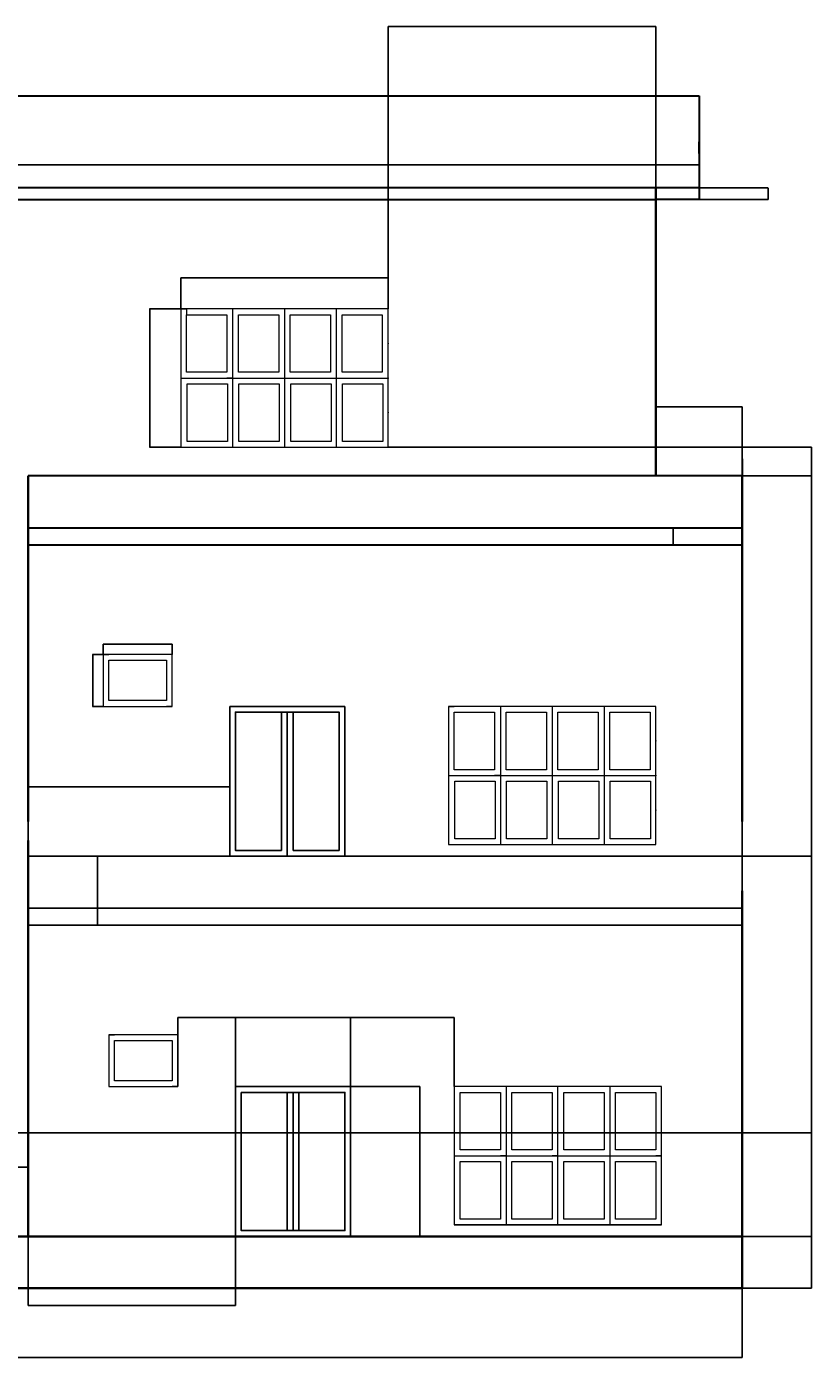
# Model space of a CAD drawing. Units: millimetres. Extents: x 54 to 12356, y 76 to 11627.
# Tile 2 of 2: x 5541 to 12356, y 76 to 11627. Entities that reach past the tile are written whole.
import ezdxf

# ---------------------------------------------------------------- set-up
doc = ezdxf.new("R2010")
doc.units = ezdxf.units.MM
for name, color, linetype, lineweight in [('A-ANNO-DIMS', 2, 'Continuous', 18), ('A-DOOR', 3, 'Continuous', 25), ('A-FLOR', 7, 'Continuous', 25), ('A-GLAZ', 4, 'Continuous', 18), ('A-GLAZ-LAYO', 8, 'Continuous', 13), ('A-ROOF', 7, 'Continuous', 30), ('A-WALL', 7, 'Continuous', 35), ('S-FNDN', 7, 'Continuous', 35)]:
    doc.layers.add(name, color=color, linetype=linetype, lineweight=lineweight)
doc.styles.get("Standard").update_dxf_attribs({"font": 'arial.ttf'})
doc.dimstyles.get("Standard").update_dxf_attribs({"dimtxt": 0.18, "dimasz": 0.18, "dimexe": 0.18, "dimexo": 0.0625, "dimgap": 0.09, "dimtad": 0, "dimtih": 1, "dimtoh": 1, "dimdec": 4, "dimzin": 0, "dimdsep": 46, "dimtxsty": 'Standard', "dimcen": 0.09, "dimadec": 0, "dimazin": 0, "dimtfac": 1, "dimtdec": 4, "dimtofl": 0, "dimtmove": 0, "dimatfit": 3, "dimfxl": 1, "dimtolj": 1, "dimtzin": 0, "dimarcsym": 0})

# ---------------------------------------------------------------- blocks, each defined once
blk = doc.blocks.new('WIN-FIXED-600x450')
for p, q in [((600.0002773238857, 450.00035733614), (0.0002773238857117, 450.00035733614)), ((0.0002773238857117, 450.00035733614), (0.0002773238857117, 0.0003573361400413)), ((0.0002773238857117, 450.00035733614), (50.00027732388571, 450.00035733614)), ((600.0002773238857, 0.0003573361400413), (600.0002773238857, 450.00035733614)), ((0.0002773238857117, 0.0003573361400413), (600.0002773238857, 0.0003573361400413)), ((600.0002773238857, 0.0003573361400413), (550.0002773238857, 0.0003573361400413))]:
    blk.add_line(p, q)
blk.add_lwpolyline([(50.00027732388571, 400.00035733614), (550.0002773238857, 400.00035733614), (550.0002773238857, 50.00035733614004), (50.00027732388571, 50.00035733614004)], close=True)
blk = doc.blocks.new('WIN-8L-1800x1200')
for p, q in [((1800.000277323883, 1200.00035733614), (0.0002773238829832, 1200.00035733614)), ((0.0002773238829832, 1200.00035733614), (0.0002773238829832, 0.0003573361400413)), ((0.0002773238829832, 1200.00035733614), (50.00027732388298, 1200.00035733614)), ((450.0002773238829, 1200.00035733614), (450.0002773238829, 0.0003573361400413)), ((900.0002773238829, 1200.00035733614), (900.0002773238829, 0.0003573361400413)), ((1350.000277323883, 1200.00035733614), (1350.000277323883, 0.0003573361400413)), ((1800.000277323883, 0.0003573361400413), (1800.000277323883, 1200.00035733614)), ((0.0002773238829832, 600.00035733614), (1800.000277323883, 600.00035733614)), ((450.0002773238829, 600.00035733614), (400.0002773238829, 600.00035733614)), ((0.0002773238829832, 0.0003573361400413), (1800.000277323883, 0.0003573361400413))]:
    blk.add_line(p, q)
for points in [[(50.00027732388298, 1150.00035733614), (400.0002773238829, 1150.00035733614), (400.0002773238829, 650.00035733614), (50.00027732388298, 650.00035733614)], [(500.0002773238829, 1150.00035733614), (850.0002773238829, 1150.00035733614), (850.0002773238829, 650.00035733614), (500.0002773238829, 650.00035733614)], [(950.0002773238829, 1150.00035733614), (1300.000277323883, 1150.00035733614), (1300.000277323883, 650.00035733614), (950.0002773238829, 650.00035733614)], [(1400.000277323883, 1150.00035733614), (1750.000277323883, 1150.00035733614), (1750.000277323883, 650.00035733614), (1400.000277323883, 650.00035733614)], [(54.55140368687716, 550.00035733614), (404.5514036868771, 550.00035733614), (404.5514036868771, 50.00035733614004), (54.55140368687716, 50.00035733614004)], [(504.5514036868771, 550.00035733614), (854.551403686877, 550.00035733614), (854.551403686877, 50.00035733614004), (504.5514036868771, 50.00035733614004)], [(954.551403686877, 550.00035733614), (1304.551403686877, 550.00035733614), (1304.551403686877, 50.00035733614004), (954.551403686877, 50.00035733614004)], [(1404.551403686877, 550.00035733614), (1754.551403686877, 550.00035733614), (1754.551403686877, 50.00035733614004), (1404.551403686877, 50.00035733614004)]]:
    blk.add_lwpolyline(points, close=True)
blk = doc.blocks.new('*D11')
at = {"layer": 'A-ANNO-DIMS', "color": 0, "lineweight": -2, "transparency": 16777216}
for p, q in [((6204.93127732388, 6176.485857336136), (6204.93127732388, 6266.603357336137)), ((6205.11127732388, 6266.423357336137), (6503.346577460305, 6266.423357336137)), ((6804.751277323879, 6266.423357336137), (6506.515977187454, 6266.423357336137)), ((6804.93127732388, 6176.485857336136), (6804.93127732388, 6266.603357336137))]:
    blk.add_line(p, q, dxfattribs=at)
at = {"layer": 'A-ANNO-DIMS', "color": 0, "transparency": 16777216}
for points in [[(6205.11127732388, 6266.453357336136), (6205.11127732388, 6266.393357336137), (6204.93127732388, 6266.423357336137)], [(6804.751277323879, 6266.453357336136), (6804.751277323879, 6266.393357336137), (6804.93127732388, 6266.423357336137)]]:
    blk.add_solid(points, dxfattribs=at)
at = {"layer": 'Defpoints', "color": 0, "transparency": 16777216}
for p in [(6804.93127732388, 6266.423357336137), (6204.93127732388, 6176.423357336137), (6804.93127732388, 6176.423357336137)]:
    blk.add_point(p, dxfattribs=at)
at = {"layer": 'A-ANNO-DIMS', "color": 0, "transparency": 16777216, "insert": (6504.93127732388, 6266.423357336137), "char_height": 0.18, "attachment_point": 5}
blk.add_mtext('\\A1;FIXED WINDOW 600 TYP.', dxfattribs=at)
blk = doc.blocks.new('*D12')
at = {"layer": 'A-ANNO-DIMS', "color": 0, "lineweight": -2, "transparency": 16777216}
for p, q in [((6204.868777323884, 6176.42335733614), (6114.751277323883, 6176.423357336139)), ((6114.931277323883, 6176.243357336138), (6114.931277323883, 5951.605260473928)), ((6114.931277323883, 5726.603357336138), (6114.931277323883, 5951.241454198348)), ((6204.868777323884, 5726.423357336138), (6114.751277323883, 5726.423357336138))]:
    blk.add_line(p, q, dxfattribs=at)
at = {"layer": 'A-ANNO-DIMS', "color": 0, "transparency": 16777216}
for points in [[(6114.901277323883, 6176.243357336138), (6114.961277323882, 6176.243357336138), (6114.931277323883, 6176.423357336139)], [(6114.901277323884, 5726.603357336138), (6114.961277323883, 5726.603357336138), (6114.931277323883, 5726.423357336138)]]:
    blk.add_solid(points, dxfattribs=at)
at = {"layer": 'Defpoints', "color": 0, "transparency": 16777216}
for p in [(6114.931277323883, 6176.423357336139), (6204.931277323884, 6176.42335733614), (6204.931277323884, 5726.423357336138)]:
    blk.add_point(p, dxfattribs=at)
at = {"layer": 'A-ANNO-DIMS', "color": 0, "transparency": 16777216, "insert": (6114.931277323883, 5951.423357336136), "char_height": 0.18, "attachment_point": 5}
blk.add_mtext('\\A1;450 TYP.', dxfattribs=at)
blk = doc.blocks.new('*D13')
at = {"layer": 'A-ANNO-DIMS', "color": 0, "lineweight": -2, "transparency": 16777216}
for p, q in [((6879.931277323887, 9176.485857336142), (6879.931277323887, 9446.603357336142)), ((6880.111277323887, 9446.423357336142), (7778.159640216109, 9446.423357336142)), ((8679.751277323887, 9446.423357336142), (7781.702914431661, 9446.423357336142)), ((8679.931277323885, 9176.485857336142), (8679.931277323885, 9446.603357336142))]:
    blk.add_line(p, q, dxfattribs=at)
at = {"layer": 'A-ANNO-DIMS', "color": 0, "transparency": 16777216}
for points in [[(6880.111277323887, 9446.453357336142), (6880.111277323887, 9446.393357336141), (6879.931277323887, 9446.423357336142)], [(8679.751277323887, 9446.453357336142), (8679.751277323887, 9446.393357336141), (8679.931277323885, 9446.423357336142)]]:
    blk.add_solid(points, dxfattribs=at)
at = {"layer": 'Defpoints', "color": 0, "transparency": 16777216}
for p in [(8679.931277323885, 9446.423357336142), (6879.931277323887, 9176.423357336142), (8679.931277323885, 9176.423357336142)]:
    blk.add_point(p, dxfattribs=at)
at = {"layer": 'A-ANNO-DIMS', "color": 0, "transparency": 16777216, "insert": (7779.931277323886, 9446.423357336142), "char_height": 0.18, "attachment_point": 5}
blk.add_mtext('\\A1;8-LIGHT WINDOW 1800 TYP.', dxfattribs=at)
blk = doc.blocks.new('*D14')
at = {"layer": 'A-ANNO-DIMS', "color": 0, "lineweight": -2, "transparency": 16777216}
for p, q in [((6879.868777323889, 9176.423357336145), (6609.751277323893, 9176.423357336145)), ((6609.931277323894, 9176.243357336145), (6609.931277323894, 8576.605260473934)), ((6609.931277323894, 7976.603357336145), (6609.931277323894, 8576.241454198356)), ((6879.868777323889, 7976.423357336145), (6609.751277323893, 7976.423357336145))]:
    blk.add_line(p, q, dxfattribs=at)
at = {"layer": 'A-ANNO-DIMS', "color": 0, "transparency": 16777216}
for points in [[(6609.901277323894, 9176.243357336145), (6609.961277323893, 9176.243357336145), (6609.931277323894, 9176.423357336145)], [(6609.901277323894, 7976.603357336145), (6609.961277323893, 7976.603357336145), (6609.931277323894, 7976.423357336145)]]:
    blk.add_solid(points, dxfattribs=at)
at = {"layer": 'Defpoints', "color": 0, "transparency": 16777216}
for p in [(6609.931277323894, 9176.423357336145), (6879.93127732389, 9176.423357336145), (6879.93127732389, 7976.423357336145)]:
    blk.add_point(p, dxfattribs=at)
at = {"layer": 'A-ANNO-DIMS', "color": 0, "transparency": 16777216, "insert": (6609.931277323894, 8576.423357336143), "char_height": 0.18, "attachment_point": 5}
blk.add_mtext('\\A1;1200 TYP.', dxfattribs=at)
blk = doc.blocks.new('*D19')
at = {"layer": 'A-ANNO-DIMS', "color": 0, "lineweight": -2, "transparency": 16777216}
for p, q in [((654.931277, 676.360857), (654.931277, 75.74335700000005)), ((11754.931277, 676.360857), (11754.931277, 75.74335700000005)), ((655.1112769999999, 75.923357), (6204.511358855389, 75.923357)), ((11754.751277, 75.923357), (6205.351195144611, 75.923357))]:
    blk.add_line(p, q, dxfattribs=at)
at = {"layer": 'A-ANNO-DIMS', "color": 0, "transparency": 16777216}
for points in [[(655.1112769999999, 75.953357), (655.1112769999999, 75.893357), (654.931277, 75.923357)], [(11754.751277, 75.953357), (11754.751277, 75.893357), (11754.931277, 75.923357)]]:
    blk.add_solid(points, dxfattribs=at)
at = {"layer": 'Defpoints', "color": 0, "transparency": 16777216}
for p in [(654.931277, 676.423357), (11754.931277, 676.423357), (11754.931277, 75.923357)]:
    blk.add_point(p, dxfattribs=at)
at = {"layer": 'A-ANNO-DIMS', "color": 0, "transparency": 16777216, "insert": (6204.931277, 75.923357), "char_height": 0.18, "attachment_point": 5}
blk.add_mtext('\\A1;11100', dxfattribs=at)
blk = doc.blocks.new('*D21')
at = {"layer": 'A-ANNO-DIMS', "color": 0, "lineweight": -2, "transparency": 16777216}
for p, q in [((2379.931277, 11026.360857), (2379.931277, 10425.743357)), ((11379.931277, 11026.360857), (11379.931277, 10425.743357)), ((2380.111277, 10425.923357), (6879.57281178854, 10425.923357)), ((11379.751277, 10425.923357), (6880.289742211459, 10425.923357))]:
    blk.add_line(p, q, dxfattribs=at)
at = {"layer": 'A-ANNO-DIMS', "color": 0, "transparency": 16777216}
for points in [[(2380.111277, 10425.953357), (2380.111277, 10425.893357), (2379.931277, 10425.923357)], [(11379.751277, 10425.953357), (11379.751277, 10425.893357), (11379.931277, 10425.923357)]]:
    blk.add_solid(points, dxfattribs=at)
at = {"layer": 'Defpoints', "color": 0, "transparency": 16777216}
for p in [(2379.931277, 11026.423357), (11379.931277, 11026.423357), (2379.931277, 10425.923357)]:
    blk.add_point(p, dxfattribs=at)
at = {"layer": 'A-ANNO-DIMS', "color": 0, "transparency": 16777216, "insert": (6879.931277, 10425.923357), "char_height": 0.18, "attachment_point": 5}
blk.add_mtext('\\A1;9000', dxfattribs=at)
blk = doc.blocks.new('*D25')
at = {"layer": 'A-ANNO-DIMS', "color": 0, "lineweight": -2, "transparency": 16777216}
for p, q in [((2754.931277, 1126.485857), (2754.931277, 1727.103357)), ((2755.111277, 1726.923357), (4154.571277, 1726.923357)), ((5554.751277, 1726.923357), (4155.291276999999, 1726.923357)), ((5554.931277, 1126.485857), (5554.931277, 1727.103357))]:
    blk.add_line(p, q, dxfattribs=at)
at = {"layer": 'A-ANNO-DIMS', "color": 0, "transparency": 16777216}
for points in [[(2755.111277, 1726.953357), (2755.111277, 1726.893356999999), (2754.931277, 1726.923357)], [(5554.751277, 1726.953357), (5554.751277, 1726.893356999999), (5554.931277, 1726.923357)]]:
    blk.add_solid(points, dxfattribs=at)
at = {"layer": 'Defpoints', "color": 0, "transparency": 16777216}
for p in [(5554.931277, 1726.923357), (2754.931277, 1126.423357), (5554.931277, 1126.423357)]:
    blk.add_point(p, dxfattribs=at)
at = {"layer": 'A-ANNO-DIMS', "color": 0, "transparency": 16777216, "insert": (4154.931277, 1726.923357), "char_height": 0.18, "attachment_point": 5}
blk.add_mtext('\\A1;2800', dxfattribs=at)
blk = doc.blocks.new('*D26')
at = {"layer": 'A-ANNO-DIMS', "color": 0, "lineweight": -2, "transparency": 16777216}
for p, q in [((11754.993777, 1126.423357), (12355.61127700001, 1126.423357)), ((12355.43127700001, 1126.243357), (12355.43127700001, 901.6052601377904)), ((12355.43127700001, 676.6033570000002), (12355.43127700001, 901.2414538622104)), ((11754.993777, 676.4233570000002), (12355.61127700001, 676.4233570000004))]:
    blk.add_line(p, q, dxfattribs=at)
at = {"layer": 'A-ANNO-DIMS', "color": 0, "transparency": 16777216}
for points in [[(12355.40127700001, 1126.243357), (12355.46127700001, 1126.243357), (12355.43127700001, 1126.423357)], [(12355.40127700001, 676.6033570000002), (12355.46127700001, 676.6033570000002), (12355.43127700001, 676.4233570000004)]]:
    blk.add_solid(points, dxfattribs=at)
at = {"layer": 'Defpoints', "color": 0, "transparency": 16777216}
for p in [(11754.931277, 1126.423357), (11754.931277, 676.4233570000002), (12355.43127700001, 676.4233570000004)]:
    blk.add_point(p, dxfattribs=at)
at = {"layer": 'A-ANNO-DIMS', "color": 0, "transparency": 16777216, "insert": (12355.43127700001, 901.4233569999968), "char_height": 0.18, "attachment_point": 5}
blk.add_mtext('\\A1;450', dxfattribs=at)
blk = doc.blocks.new('*D27')
at = {"layer": 'A-ANNO-DIMS', "color": 0, "lineweight": -2, "transparency": 16777216}
for p, q in [((11754.993777, 4426.423357000001), (12355.61127700001, 4426.423357000001)), ((12355.43127700001, 4426.243357000001), (12355.43127700001, 2776.605321529333)), ((12355.43127700001, 1126.603357), (12355.43127700001, 2776.241392470669)), ((11754.993777, 1126.423357), (12355.61127700001, 1126.423357))]:
    blk.add_line(p, q, dxfattribs=at)
at = {"layer": 'A-ANNO-DIMS', "color": 0, "transparency": 16777216}
for points in [[(12355.40127700001, 4426.243357000001), (12355.46127700001, 4426.243357000001), (12355.43127700001, 4426.423357000001)], [(12355.40127700001, 1126.603357), (12355.46127700001, 1126.603357), (12355.43127700001, 1126.423357)]]:
    blk.add_solid(points, dxfattribs=at)
at = {"layer": 'Defpoints', "color": 0, "transparency": 16777216}
for p in [(11754.931277, 4426.423357000001), (11754.931277, 1126.423357), (12355.43127700001, 1126.423357)]:
    blk.add_point(p, dxfattribs=at)
at = {"layer": 'A-ANNO-DIMS', "color": 0, "transparency": 16777216, "insert": (12355.43127700001, 2776.423356999997), "char_height": 0.18, "attachment_point": 5}
blk.add_mtext('\\A1;3300', dxfattribs=at)
blk = doc.blocks.new('*D28')
at = {"layer": 'A-ANNO-DIMS', "color": 0, "lineweight": -2, "transparency": 16777216}
for p, q in [((11754.993777, 7726.423357000003), (12355.61127700001, 7726.423357000003)), ((12355.43127700001, 7726.243357000003), (12355.43127700001, 6076.605321529333)), ((12355.43127700001, 4426.603357000002), (12355.43127700001, 6076.24139247067)), ((11754.993777, 4426.423357000001), (12355.61127700001, 4426.423357000001))]:
    blk.add_line(p, q, dxfattribs=at)
at = {"layer": 'A-ANNO-DIMS', "color": 0, "transparency": 16777216}
for points in [[(12355.40127700001, 7726.243357000003), (12355.46127700001, 7726.243357000003), (12355.43127700001, 7726.423357000003)], [(12355.40127700001, 4426.603357000002), (12355.46127700001, 4426.603357000002), (12355.43127700001, 4426.423357000001)]]:
    blk.add_solid(points, dxfattribs=at)
at = {"layer": 'Defpoints', "color": 0, "transparency": 16777216}
for p in [(11754.931277, 7726.423357000003), (11754.931277, 4426.423357000001), (12355.43127700001, 4426.423357000001)]:
    blk.add_point(p, dxfattribs=at)
at = {"layer": 'A-ANNO-DIMS', "color": 0, "transparency": 16777216, "insert": (12355.43127700001, 6076.423356999997), "char_height": 0.18, "attachment_point": 5}
blk.add_mtext('\\A1;3300', dxfattribs=at)
blk = doc.blocks.new('*D29')
at = {"layer": 'A-ANNO-DIMS', "color": 0, "lineweight": -2, "transparency": 16777216}
for p, q in [((5554.993777000001, 4426.423357000001), (6155.611277000008, 4426.423357000002)), ((6155.431277000007, 4426.243357000002), (6155.431277000007, 4126.605260137792)), ((6155.431277000007, 3826.603357000002), (6155.431277000007, 4126.241453862212)), ((5554.993777000001, 3826.423357000003), (6155.611277000008, 3826.423357000003))]:
    blk.add_line(p, q, dxfattribs=at)
at = {"layer": 'A-ANNO-DIMS', "color": 0, "transparency": 16777216}
for points in [[(6155.401277000007, 4426.243357000002), (6155.461277000007, 4426.243357000002), (6155.431277000007, 4426.423357000002)], [(6155.401277000007, 3826.603357000002), (6155.461277000007, 3826.603357000002), (6155.431277000007, 3826.423357000003)]]:
    blk.add_solid(points, dxfattribs=at)
at = {"layer": 'Defpoints', "color": 0, "transparency": 16777216}
for p in [(5554.931277000001, 4426.423357000001), (5554.931277000001, 3826.423357000003), (6155.431277000007, 3826.423357000003)]:
    blk.add_point(p, dxfattribs=at)
at = {"layer": 'A-ANNO-DIMS', "color": 0, "transparency": 16777216, "insert": (6155.431277000006, 4126.423356999999), "char_height": 0.18, "attachment_point": 5}
blk.add_mtext('\\A1;600', dxfattribs=at)
blk = doc.blocks.new('*D30')
at = {"layer": 'A-ANNO-DIMS', "color": 0, "lineweight": -2, "transparency": 16777216}
for p, q in [((11754.868777, 7276.423357000003), (11154.251277, 7276.423357000003)), ((11154.431277, 7276.243357000002), (11154.431277, 7201.605260137793)), ((11154.431277, 7126.603357000004), (11154.431277, 7201.241453862214)), ((11754.868777, 7126.423357000003), (11154.251277, 7126.423357000003))]:
    blk.add_line(p, q, dxfattribs=at)
at = {"layer": 'A-ANNO-DIMS', "color": 0, "transparency": 16777216}
for points in [[(11154.40127700001, 7276.243357000002), (11154.461277, 7276.243357000002), (11154.431277, 7276.423357000003)], [(11154.40127700001, 7126.603357000004), (11154.461277, 7126.603357000004), (11154.431277, 7126.423357000003)]]:
    blk.add_solid(points, dxfattribs=at)
at = {"layer": 'Defpoints', "color": 0, "transparency": 16777216}
for p in [(11154.431277, 7276.423357000003), (11754.931277, 7276.423357000003), (11754.931277, 7126.423357000003)]:
    blk.add_point(p, dxfattribs=at)
at = {"layer": 'A-ANNO-DIMS', "color": 0, "transparency": 16777216, "insert": (11154.431277, 7201.423356999997), "char_height": 0.18, "attachment_point": 5}
blk.add_mtext('\\A1;150', dxfattribs=at)
blk = doc.blocks.new('*D31')
at = {"layer": 'A-ANNO-DIMS', "color": 0, "lineweight": -2, "transparency": 16777216}
for p, q in [((11004.931277, 7726.485857), (11004.931277, 8327.103357)), ((11005.111277, 8326.923357), (11379.64347345293, 8326.923357)), ((11754.751277, 8326.923357), (11380.21908054706, 8326.923357)), ((11754.931277, 7726.485857), (11754.931277, 8327.103357))]:
    blk.add_line(p, q, dxfattribs=at)
at = {"layer": 'A-ANNO-DIMS', "color": 0, "transparency": 16777216}
for points in [[(11005.111277, 8326.953357), (11005.111277, 8326.893356999999), (11004.931277, 8326.923357)], [(11754.751277, 8326.953357), (11754.751277, 8326.893356999999), (11754.931277, 8326.923357)]]:
    blk.add_solid(points, dxfattribs=at)
at = {"layer": 'Defpoints', "color": 0, "transparency": 16777216}
for p in [(11754.931277, 8326.923357), (11004.931277, 7726.423357), (11754.931277, 7726.423357)]:
    blk.add_point(p, dxfattribs=at)
at = {"layer": 'A-ANNO-DIMS', "color": 0, "transparency": 16777216, "insert": (11379.931277, 8326.923357), "char_height": 0.18, "attachment_point": 5}
blk.add_mtext('\\A1;750', dxfattribs=at)
blk = doc.blocks.new('*D32')
at = {"layer": 'A-ANNO-DIMS', "color": 0, "lineweight": -2, "transparency": 16777216}
for p, q in [((8679.931277, 9176.485857000001), (8679.931277, 11627.103357)), ((8680.111276999998, 11626.923357), (9842.070294735337, 11626.923357)), ((11004.751277, 11626.923357), (9842.792259264665, 11626.923357)), ((11004.931277, 10226.485857), (11004.931277, 11627.103357))]:
    blk.add_line(p, q, dxfattribs=at)
at = {"layer": 'A-ANNO-DIMS', "color": 0, "transparency": 16777216}
for points in [[(8680.111276999998, 11626.953357), (8680.111276999998, 11626.893357), (8679.931277, 11626.923357)], [(11004.751277, 11626.953357), (11004.751277, 11626.893357), (11004.931277, 11626.923357)]]:
    blk.add_solid(points, dxfattribs=at)
at = {"layer": 'Defpoints', "color": 0, "transparency": 16777216}
for p in [(8679.931277, 11626.923357), (11004.931277, 10226.423357), (8679.931277, 9176.423357)]:
    blk.add_point(p, dxfattribs=at)
at = {"layer": 'A-ANNO-DIMS', "color": 0, "transparency": 16777216, "insert": (9842.431277000002, 11626.923357), "char_height": 0.18, "attachment_point": 5}
blk.add_mtext('\\A1;2325', dxfattribs=at)
blk = doc.blocks.new('*D33')
at = {"layer": 'A-ANNO-DIMS', "color": 0, "lineweight": -2, "transparency": 16777216}
for p, q in [((8679.993777000003, 7976.423357000003), (12355.61127700001, 7976.423357000005)), ((12355.43127700001, 7976.243357000004), (12355.43127700001, 7851.605260137795)), ((12355.43127700001, 7726.603357000003), (12355.43127700001, 7851.241453862214)), ((11754.993777, 7726.423357000003), (12355.61127700001, 7726.423357000003))]:
    blk.add_line(p, q, dxfattribs=at)
at = {"layer": 'A-ANNO-DIMS', "color": 0, "transparency": 16777216}
for points in [[(12355.40127700001, 7976.243357000004), (12355.46127700001, 7976.243357000004), (12355.43127700001, 7976.423357000005)], [(12355.40127700001, 7726.603357000003), (12355.46127700001, 7726.603357000003), (12355.43127700001, 7726.423357000003)]]:
    blk.add_solid(points, dxfattribs=at)
at = {"layer": 'Defpoints', "color": 0, "transparency": 16777216}
for p in [(8679.931277000003, 7976.423357000003), (11754.931277, 7726.423357000003), (12355.43127700001, 7726.423357000003)]:
    blk.add_point(p, dxfattribs=at)
at = {"layer": 'A-ANNO-DIMS', "color": 0, "transparency": 16777216, "insert": (12355.43127700001, 7851.423356999998), "char_height": 0.18, "attachment_point": 5}
blk.add_mtext('\\A1;250', dxfattribs=at)
blk = doc.blocks.new('*D37')
at = {"layer": 'A-ANNO-DIMS', "color": 0, "lineweight": -2, "transparency": 16777216}
for p, q in [((4926.802842000002, 2025.286183000001), (12355.61127700001, 2025.286183000002)), ((12355.43127700001, 2025.106183000002), (12355.43127700001, 1576.036673137792)), ((12355.43127700001, 1126.603357000002), (12355.43127700001, 1575.672866862212)), ((2754.993777000001, 1126.423357), (12355.61127700001, 1126.423357000001))]:
    blk.add_line(p, q, dxfattribs=at)
at = {"layer": 'A-ANNO-DIMS', "color": 0, "transparency": 16777216}
for points in [[(12355.40127700001, 2025.106183000002), (12355.46127700001, 2025.106183000002), (12355.43127700001, 2025.286183000002)], [(12355.40127700001, 1126.603357000002), (12355.46127700001, 1126.603357000002), (12355.43127700001, 1126.423357000001)]]:
    blk.add_solid(points, dxfattribs=at)
at = {"layer": 'Defpoints', "color": 0, "transparency": 16777216}
for p in [(4926.740342000002, 2025.286183000001), (12355.43127700001, 2025.286183000002), (2754.931277000001, 1126.423357)]:
    blk.add_point(p, dxfattribs=at)
at = {"layer": 'A-ANNO-DIMS', "color": 0, "transparency": 16777216, "insert": (12355.43127700001, 1575.854769999998), "char_height": 0.18, "attachment_point": 5}
blk.add_mtext('\\A1;898.9', dxfattribs=at)
blk = doc.blocks.new('*D38')
at = {"layer": 'A-ANNO-DIMS', "color": 0, "lineweight": -2, "transparency": 16777216}
for p, q in [((5554.931277, 1126.360857), (5554.931277, 525.743357)), ((7354.931277, 1126.360857), (7354.931277, 525.743357)), ((5555.111277, 525.923357), (6454.581283821283, 525.923357)), ((7354.751277, 525.923357), (6455.281270178717, 525.923357))]:
    blk.add_line(p, q, dxfattribs=at)
at = {"layer": 'A-ANNO-DIMS', "color": 0, "transparency": 16777216}
for points in [[(5555.111277, 525.953357), (5555.111277, 525.893357), (5554.931277, 525.923357)], [(7354.751277, 525.953357), (7354.751277, 525.893357), (7354.931277, 525.923357)]]:
    blk.add_solid(points, dxfattribs=at)
at = {"layer": 'Defpoints', "color": 0, "transparency": 16777216}
for p in [(5554.931277, 1126.423357), (7354.931277, 1126.423357), (5554.931277, 525.923357)]:
    blk.add_point(p, dxfattribs=at)
at = {"layer": 'A-ANNO-DIMS', "color": 0, "transparency": 16777216, "insert": (6454.931277, 525.923357), "char_height": 0.18, "attachment_point": 5}
blk.add_mtext('\\A1;1800', dxfattribs=at)
blk = doc.blocks.new('*D39')
at = {"layer": 'A-ANNO-DIMS', "color": 0, "lineweight": -2, "transparency": 16777216}
for p, q in [((6854.931277, 2426.485857), (6854.931277, 3027.103357)), ((6855.111277, 3026.923357), (7104.642736754434, 3026.923357)), ((7354.751277, 3026.923357), (7105.219817245566, 3026.923357)), ((7354.931277, 2426.485857), (7354.931277, 3027.103357))]:
    blk.add_line(p, q, dxfattribs=at)
at = {"layer": 'A-ANNO-DIMS', "color": 0, "transparency": 16777216}
for points in [[(6855.111277, 3026.953357), (6855.111277, 3026.893357), (6854.931277, 3026.923357)], [(7354.751277, 3026.953357), (7354.751277, 3026.893357), (7354.931277, 3026.923357)]]:
    blk.add_solid(points, dxfattribs=at)
at = {"layer": 'Defpoints', "color": 0, "transparency": 16777216}
for p in [(7354.931277, 3026.923357), (6854.931277, 2426.423357), (7354.931277, 2426.423357)]:
    blk.add_point(p, dxfattribs=at)
at = {"layer": 'A-ANNO-DIMS', "color": 0, "transparency": 16777216, "insert": (7104.931277, 3026.923357), "char_height": 0.18, "attachment_point": 5}
blk.add_mtext('\\A1;500', dxfattribs=at)
blk = doc.blocks.new('*D40')
at = {"layer": 'A-ANNO-DIMS', "color": 0, "lineweight": -2, "transparency": 16777216}
for p, q in [((7354.931277, 2426.485857), (7354.931277, 3027.103357)), ((7355.111277, 3026.923357), (7854.581283821282, 3026.923357)), ((8354.751277, 3026.923357), (7855.281270178718, 3026.923357)), ((8354.931277, 2426.485857), (8354.931277, 3027.103357))]:
    blk.add_line(p, q, dxfattribs=at)
at = {"layer": 'A-ANNO-DIMS', "color": 0, "transparency": 16777216}
for points in [[(7355.111277, 3026.953357), (7355.111277, 3026.893357), (7354.931277, 3026.923357)], [(8354.751277, 3026.953357), (8354.751277, 3026.893357), (8354.931277, 3026.923357)]]:
    blk.add_solid(points, dxfattribs=at)
at = {"layer": 'Defpoints', "color": 0, "transparency": 16777216}
for p in [(8354.931277, 3026.923357), (7354.931277, 2426.423357), (8354.931277, 2426.423357)]:
    blk.add_point(p, dxfattribs=at)
at = {"layer": 'A-ANNO-DIMS', "color": 0, "transparency": 16777216, "insert": (7854.931277, 3026.923357), "char_height": 0.18, "attachment_point": 5}
blk.add_mtext('\\A1;1000', dxfattribs=at)
blk = doc.blocks.new('*D41')
at = {"layer": 'A-ANNO-DIMS', "color": 0, "lineweight": -2, "transparency": 16777216}
for p, q in [((8354.931277, 2426.485857), (8354.931277, 3027.103357)), ((8355.111277, 3026.923357), (8804.642736754431, 3026.923357)), ((9254.751277, 3026.923357), (8805.219817245566, 3026.923357)), ((9254.931277, 2426.485857), (9254.931277, 3027.103357))]:
    blk.add_line(p, q, dxfattribs=at)
at = {"layer": 'A-ANNO-DIMS', "color": 0, "transparency": 16777216}
for points in [[(8355.111277, 3026.953357), (8355.111277, 3026.893357), (8354.931277, 3026.923357)], [(9254.751277, 3026.953357), (9254.751277, 3026.893357), (9254.931277, 3026.923357)]]:
    blk.add_solid(points, dxfattribs=at)
at = {"layer": 'Defpoints', "color": 0, "transparency": 16777216}
for p in [(9254.931277, 3026.923357), (8354.931277, 2426.423357), (9254.931277, 2426.423357)]:
    blk.add_point(p, dxfattribs=at)
at = {"layer": 'A-ANNO-DIMS', "color": 0, "transparency": 16777216, "insert": (8804.931277, 3026.923357), "char_height": 0.18, "attachment_point": 5}
blk.add_mtext('\\A1;900', dxfattribs=at)
blk = doc.blocks.new('*D42')
at = {"layer": 'A-ANNO-DIMS', "color": 0, "lineweight": -2, "transparency": 16777216}
for p, q in [((8354.993777000002, 2426.423357000001), (8955.611277000007, 2426.423357000001)), ((8955.431277000007, 2426.243357000001), (8955.431277000007, 1776.605321529333)), ((8955.431277000007, 1126.603357), (8955.431277000007, 1776.24139247067)), ((8354.993777000002, 1126.423357), (8955.611277000007, 1126.423357))]:
    blk.add_line(p, q, dxfattribs=at)
at = {"layer": 'A-ANNO-DIMS', "color": 0, "transparency": 16777216}
for points in [[(8955.401277000006, 2426.243357000001), (8955.461277000008, 2426.243357000001), (8955.431277000007, 2426.423357000001)], [(8955.401277000006, 1126.603357), (8955.461277000008, 1126.603357), (8955.431277000007, 1126.423357)]]:
    blk.add_solid(points, dxfattribs=at)
at = {"layer": 'Defpoints', "color": 0, "transparency": 16777216}
for p in [(8354.931277000003, 2426.423357000001), (8354.931277000003, 1126.423357), (8955.431277000007, 1126.423357)]:
    blk.add_point(p, dxfattribs=at)
at = {"layer": 'A-ANNO-DIMS', "color": 0, "transparency": 16777216, "insert": (8955.431277000005, 1776.423356999998), "char_height": 0.18, "attachment_point": 5}
blk.add_mtext('\\A1;1300', dxfattribs=at)
blk = doc.blocks.new('*D43')
at = {"layer": 'A-ANNO-DIMS', "color": 0, "lineweight": -2, "transparency": 16777216}
for p, q in [((5554.931277, 4426.485856999999), (5554.931277, 5027.103357)), ((5555.111277, 5026.923357), (6429.581283821282, 5026.923357)), ((7304.751277, 5026.923357), (6430.281270178717, 5026.923357)), ((7304.931277, 4426.485856999999), (7304.931277, 5027.103357))]:
    blk.add_line(p, q, dxfattribs=at)
at = {"layer": 'A-ANNO-DIMS', "color": 0, "transparency": 16777216}
for points in [[(5555.111277, 5026.953357), (5555.111277, 5026.893357), (5554.931277, 5026.923357)], [(7304.751277, 5026.953357), (7304.751277, 5026.893357), (7304.931277, 5026.923357)]]:
    blk.add_solid(points, dxfattribs=at)
at = {"layer": 'Defpoints', "color": 0, "transparency": 16777216}
for p in [(7304.931277, 5026.923357), (5554.931277, 4426.423357), (7304.931277, 4426.423357)]:
    blk.add_point(p, dxfattribs=at)
at = {"layer": 'A-ANNO-DIMS', "color": 0, "transparency": 16777216, "insert": (6429.931277, 5026.923357), "char_height": 0.18, "attachment_point": 5}
blk.add_mtext('\\A1;1750', dxfattribs=at)
blk = doc.blocks.new('*D47')
at = {"layer": 'A-ANNO-DIMS', "color": 0, "lineweight": -2, "transparency": 16777216}
for p, q in [((11379.993777, 10226.423357), (11980.61127700001, 10226.423357)), ((11980.431277, 10226.243357), (11980.431277, 10176.60526013779)), ((11980.431277, 10126.603357), (11980.431277, 10176.24145386221)), ((11379.993777, 10126.423357), (11980.61127700001, 10126.423357))]:
    blk.add_line(p, q, dxfattribs=at)
at = {"layer": 'A-ANNO-DIMS', "color": 0, "transparency": 16777216}
for points in [[(11980.40127700001, 10226.243357), (11980.461277, 10226.243357), (11980.431277, 10226.423357)], [(11980.40127700001, 10126.603357), (11980.461277, 10126.603357), (11980.431277, 10126.423357)]]:
    blk.add_solid(points, dxfattribs=at)
at = {"layer": 'Defpoints', "color": 0, "transparency": 16777216}
for p in [(11379.931277, 10226.423357), (11379.931277, 10126.423357), (11980.431277, 10126.423357)]:
    blk.add_point(p, dxfattribs=at)
at = {"layer": 'A-ANNO-DIMS', "color": 0, "transparency": 16777216, "insert": (11980.431277, 10176.423357), "char_height": 0.18, "attachment_point": 5}
blk.add_mtext('\\A1;100', dxfattribs=at)

msp = doc.modelspace()

# ---------------------------------------------------------------- linework, layer by layer
at = {"layer": 'A-DOOR'}
for p, q in [((8304.931277323883, 5726.42335733614), (7304.931277323884, 5726.42335733614)), ((7304.931277323884, 5726.42335733614), (7304.931277323882, 4426.42335733614)), ((7304.931277323884, 5726.42335733614), (7354.931277323884, 5726.42335733614)), ((7754.931277323883, 5676.42335733614), (7754.931277323883, 4476.42335733614)), ((7804.931277323884, 5676.42335733614), (7804.931277323884, 4476.42335733614)), ((7854.931277323884, 5676.42335733614), (7854.931277323884, 4476.42335733614)), ((8304.931277323883, 4426.42335733614), (8304.931277323883, 5726.42335733614)), ((7804.931277323884, 4476.42335733614), (7804.931277323884, 4426.42335733614)), ((8304.931277323883, 4426.42335733614), (8254.931277323883, 4426.42335733614)), ((8354.931277323885, 2426.42335733614), (7354.931277323885, 2426.42335733614)), ((7354.931277323885, 2426.42335733614), (7354.931277323885, 1126.42335733614)), ((7354.931277323885, 2426.42335733614), (7854.931277323885, 2426.42335733614)), ((7354.931277323885, 2426.42335733614), (7404.931277323886, 2426.42335733614)), ((7854.931277323885, 2426.42335733614), (7904.931277323886, 2426.42335733614)), ((8354.931277323885, 2326.42335733614), (8354.931277323885, 2426.42335733614)), ((7804.931277323885, 2376.42335733614), (7904.931277323886, 2376.42335733614)), ((7854.931277323885, 2376.42335733614), (7854.931277323885, 1176.42335733614)), ((8354.931277323885, 1126.42335733614), (8354.931277323885, 2326.42335733614)), ((7904.931277323886, 1176.42335733614), (7804.931277323885, 1176.42335733614)), ((7854.931277323885, 1126.42335733614), (7804.931277323885, 1126.42335733614)), ((8354.931277323885, 1126.42335733614), (8304.931277323885, 1126.42335733614))]:
    msp.add_line(p, q, dxfattribs=at)
msp.add_lwpolyline([(7754.931277323883, 4476.42335733614), (7354.931277323884, 4476.42335733614), (7354.931277323884, 5676.42335733614), (8254.931277323883, 5676.42335733614), (8254.931277323883, 4476.42335733614), (7854.931277323884, 4476.42335733614)], dxfattribs=at)
for points in [[(7404.931277323886, 2376.42335733614), (7804.931277323885, 2376.42335733614), (7804.931277323885, 1176.42335733614), (7404.931277323886, 1176.42335733614)], [(7904.931277323886, 2376.42335733614), (8304.931277323885, 2376.42335733614), (8304.931277323885, 1176.42335733614), (7904.931277323886, 1176.42335733614)]]:
    msp.add_lwpolyline(points, close=True, dxfattribs=at)
at = {"layer": 'A-FLOR'}
for p, q in [((5554.931277323885, 4276.42335733614), (5554.931277323885, 4726.42335733614)), ((11754.93127732388, 4726.42335733614), (11754.93127732388, 4276.42335733614)), ((5554.931277323885, 4426.42335733614), (11754.93127732388, 4426.42335733614)), ((9204.931277323883, 4426.42335733614), (8304.931277323883, 4426.42335733614)), ((11754.93127732388, 4426.42335733614), (11004.93127732388, 4426.42335733614)), ((11754.93127732388, 4126.42335733614), (11754.93127732388, 4276.42335733614)), ((5554.931277323885, 4026.42335733614), (5554.931277323885, 3926.42335733614)), ((11754.93127732388, 3976.42335733614), (5554.931277323885, 3976.42335733614)), ((5554.931277323885, 3926.42335733614), (5554.931277323885, 3826.42335733614)), ((5554.931277323885, 3826.42335733614), (11754.93127732388, 3826.42335733614))]:
    msp.add_line(p, q, dxfattribs=at)
at = {"layer": 'A-GLAZ'}
for p, q in [((8679.931277323883, 9176.42335733614), (6879.931277323883, 9176.42335733614)), ((6879.931277323883, 9176.42335733614), (6879.931277323883, 7976.423357336138)), ((6879.931277323883, 9176.42335733614), (6929.931277323884, 9176.42335733614)), ((6929.931277323884, 9176.42335733614), (6929.931277323884, 9126.423357336138)), ((8679.931277323883, 7976.423357336138), (8679.931277323883, 9176.42335733614)), ((11054.93127732388, 2426.42335733614), (9254.931277323885, 2426.42335733614)), ((9254.931277323885, 2426.42335733614), (9254.931277323885, 1226.42335733614)), ((9704.931277323885, 2426.42335733614), (9704.931277323885, 1226.42335733614)), ((10154.93127732388, 1226.42335733614), (10154.93127732388, 2426.42335733614)), ((10604.93127732388, 2426.42335733614), (10604.93127732388, 1226.42335733614)), ((11054.93127732388, 1226.42335733614), (11054.93127732388, 2426.42335733614)), ((9254.931277323885, 1826.42335733614), (11054.93127732388, 1826.42335733614)), ((9704.931277323885, 1826.42335733614), (9654.931277323885, 1826.42335733614)), ((10154.93127732388, 1826.42335733614), (10104.93127732388, 1826.42335733614)), ((11054.93127732388, 1826.42335733614), (11004.93127732388, 1826.42335733614)), ((9254.931277323885, 1226.42335733614), (11054.93127732388, 1226.42335733614)), ((11054.93127732388, 1226.42335733614), (9254.931277323885, 1226.42335733614)), ((9704.931277323885, 1226.42335733614), (10154.93127732388, 1226.42335733614))]:
    msp.add_line(p, q, dxfattribs=at)
for points in [[(9304.931277323885, 2376.42335733614), (9654.931277323885, 2376.42335733614), (9654.931277323885, 1876.42335733614), (9304.931277323885, 1876.42335733614)], [(9754.931277323885, 2376.42335733614), (10104.93127732388, 2376.42335733614), (10104.93127732388, 1876.42335733614), (9754.931277323885, 1876.42335733614)], [(10204.93127732388, 2376.42335733614), (10554.93127732388, 2376.42335733614), (10554.93127732388, 1876.42335733614), (10204.93127732388, 1876.42335733614)], [(10654.93127732388, 2376.42335733614), (11004.93127732388, 2376.42335733614), (11004.93127732388, 1876.42335733614), (10654.93127732388, 1876.42335733614)], [(9304.931277323885, 1776.42335733614), (9654.931277323885, 1776.42335733614), (9654.931277323885, 1276.42335733614), (9304.931277323885, 1276.42335733614)], [(9754.931277323885, 1776.42335733614), (10104.93127732388, 1776.42335733614), (10104.93127732388, 1276.42335733614), (9754.931277323885, 1276.42335733614)], [(10554.93127732388, 1276.42335733614), (10204.93127732388, 1276.42335733614), (10204.93127732388, 1776.42335733614), (10554.93127732388, 1776.42335733614)], [(11004.93127732388, 1276.42335733614), (10654.93127732388, 1276.42335733614), (10654.93127732388, 1776.42335733614), (11004.93127732388, 1776.42335733614)]]:
    msp.add_lwpolyline(points, close=True, dxfattribs=at)
at = {"layer": 'A-GLAZ-LAYO'}
for p in [(7329.931277323884, 9176.42335733614), (7779.931277323884, 9176.42335733614), (8229.931277323883, 9176.42335733614), (8679.931277323883, 8876.423357336138), (8679.931277323883, 8576.423357336136), (8679.931277323883, 8276.423357336138), (9654.931277323883, 5726.42335733614), (10104.93127732388, 5726.42335733614), (10554.93127732388, 5726.42335733614), (11004.93127732388, 5426.42335733614), (11004.93127732388, 5126.42335733614), (11004.93127732388, 4826.42335733614), (9704.931277323885, 2426.42335733614), (10154.93127732388, 2426.42335733614), (10604.93127732388, 2426.42335733614), (9704.931277323885, 1226.42335733614), (10154.93127732388, 1226.42335733614), (10604.93127732388, 1226.42335733614)]:
    msp.add_point(p, dxfattribs=at)
at = {"layer": 'A-ROOF'}
for p, q in [((2379.931277323882, 11026.42335733614), (11379.93127732388, 11026.42335733614)), ((11379.93127732388, 11026.42335733614), (11379.93127732388, 10226.42335733614)), ((11379.93127732388, 10526.42335733614), (11379.93127732388, 10626.42335733614)), ((11379.93127732388, 10226.42335733614), (2379.931277323882, 10226.42335733614)), ((11379.93127732388, 10226.42335733614), (11379.93127732388, 10126.42335733614)), ((2379.931277323882, 10126.42335733614), (11004.93127732388, 10126.42335733614)), ((11379.93127732388, 10126.42335733614), (11004.93127732388, 10126.42335733614)), ((11754.93127732388, 7876.42335733614), (11754.93127732388, 7726.423357336139)), ((11754.93127732388, 7726.423357336138), (5554.931277323884, 7726.423357336138)), ((5554.931277323884, 7726.423357336138), (5554.931277323884, 7526.423357336138)), ((5554.931277323884, 7526.423357336136), (5554.931277323884, 7126.423357336136)), ((5554.931277323884, 7276.423357336138), (11754.93127732388, 7276.423357336138)), ((11754.93127732388, 7126.423357336138), (5554.931277323884, 7126.423357336136))]:
    msp.add_line(p, q, dxfattribs=at)
at = {"layer": 'A-WALL'}
for p, q in [((11004.93127732388, 7726.423357336138), (11004.93127732388, 10226.42335733614)), ((5554.931277323885, 4726.42335733614), (5554.931277323885, 7726.423357336139)), ((11754.93127732388, 4726.42335733614), (11754.93127732388, 7726.423357336139)), ((5554.931277323885, 1126.42335733614), (5554.931277323885, 4563.351138386444)), ((5554.931277323885, 1126.42335733614), (5554.931277323885, 4126.42335733614)), ((11754.93127732388, 4126.42335733614), (11754.93127732388, 1126.42335733614)), ((11754.93127732388, 1126.42335733614), (11754.93127732388, 4126.42335733614))]:
    msp.add_line(p, q, dxfattribs=at)
at = {"layer": 'S-FNDN'}
for p, q in [((2754.931277323886, 1126.42335733614), (11754.93127732388, 1126.42335733614)), ((4954.931277323885, 1126.42335733614), (5554.931277323885, 1126.42335733614)), ((9254.931277323885, 1126.42335733614), (8354.931277323885, 1126.42335733614)), ((11754.93127732388, 1126.42335733614), (11054.93127732388, 1126.42335733614)), ((11754.93127732388, 1126.42335733614), (11754.93127732388, 676.4233573361398)), ((11754.93127732388, 676.4233573361398), (2754.931277323886, 676.4233573361398))]:
    msp.add_line(p, q, dxfattribs=at)

# ---------------------------------------------------------------- block references
at = {"layer": 'A-GLAZ'}
for name, p in [('WIN-8L-1800x1200', (6879.931000000003, 7976.423000000001)), ('WIN-FIXED-600x450', (6204.930999999994, 5726.422999999996)), ('WIN-8L-1800x1200', (9204.931, 4526.423)), ('WIN-FIXED-600x450', (6254.931, 2426.423))]:
    msp.add_blockref(name, p, dxfattribs=at)

# ---------------------------------------------------------------- dimensions: what is measured, and where the dimension line sits
at = {"layer": 'A-ANNO-DIMS'}
for base, p1, p2, picture, middle in [((8679.931277, 11626.923357), (11004.931277, 10226.423357), (8679.931277, 9176.423357), '*D32', (9842.431277000002, 11626.923357)), ((11754.931277, 8326.923357), (11004.931277, 7726.423357), (11754.931277, 7726.423357), '*D31', (11379.931277, 8326.923357)), ((7304.931277, 5026.923357), (5554.931277, 4426.423357), (7304.931277, 4426.423357), '*D43', (6429.931277, 5026.923357)), ((7354.931277, 3026.923357), (6854.931277, 2426.423357), (7354.931277, 2426.423357), '*D39', (7104.931277, 3026.923357)), ((8354.931277, 3026.923357), (7354.931277, 2426.423357), (8354.931277, 2426.423357), '*D40', (7854.931277, 3026.923357)), ((9254.931277, 3026.923357), (8354.931277, 2426.423357), (9254.931277, 2426.423357), '*D41', (8804.931277, 3026.923357)), ((5554.931277, 1726.923357), (2754.931277, 1126.423357), (5554.931277, 1126.423357), '*D25', (4154.931277, 1726.923357)), ((11754.931277, 75.923357), (654.931277, 676.423357), (11754.931277, 676.423357), '*D19', (6204.931277, 75.923357))]:
    dim = msp.add_linear_dim(base=base, p1=p1, p2=p2, dimstyle='Standard', override={"dimdec": 0, "dimlfac": 1, "dimrnd": 0, "dimzin": 0, "dimdsep": 46, "dimlunit": 2}, dxfattribs=at)
    dim.commit()
    dim.dimension.update_dxf_attribs({"geometry": picture, "text_midpoint": middle})
for base, p1, p2, angle, override, picture, middle in [((2379.931277, 10425.923357), (11379.931277, 11026.423357), (2379.931277, 11026.423357), 180, {"dimdec": 0, "dimlfac": 1, "dimrnd": 0, "dimzin": 0, "dimdsep": 46, "dimlunit": 2}, '*D21', (6879.931277, 10425.923357)), ((11980.431277, 10126.423357), (11379.931277, 10226.423357), (11379.931277, 10126.423357), 270, {"dimdec": 0, "dimlfac": 1, "dimrnd": 0, "dimzin": 0, "dimdsep": 46, "dimlunit": 2}, '*D47', (11980.431277, 10176.423357)), ((12355.43127700001, 7726.423357000003), (8679.931277, 7976.423357), (11754.931277, 7726.423357), 90, {"dimdec": 0, "dimlfac": 1, "dimrnd": 0, "dimzin": 0, "dimdsep": 46, "dimlunit": 2}, '*D33', (12355.43127700001, 7851.423356999998)), ((12355.43127700001, 4426.423357000001), (11754.931277, 7726.423357), (11754.931277, 4426.423357), 270, {"dimdec": 0, "dimlfac": 1, "dimrnd": 0, "dimzin": 0, "dimdsep": 46, "dimlunit": 2}, '*D28', (12355.43127700001, 6076.423356999997)), ((11154.431277, 7276.423357000003), (11754.931277, 7126.423357), (11754.931277, 7276.423357), 90, {"dimdec": 0, "dimlfac": 1, "dimrnd": 0, "dimzin": 0, "dimdsep": 46, "dimlunit": 2}, '*D30', (11154.431277, 7201.423356999997)), ((6155.431277000007, 3826.423357000003), (5554.931277, 4426.423357), (5554.931277, 3826.423357), 270, {"dimdec": 0, "dimlfac": 1, "dimrnd": 0, "dimzin": 0, "dimdsep": 46, "dimlunit": 2}, '*D29', (6155.431277000006, 4126.423356999999)), ((12355.43127700001, 1126.423357), (11754.931277, 4426.423357), (11754.931277, 1126.423357), 270, {"dimdec": 0, "dimlfac": 1, "dimrnd": 0, "dimzin": 0, "dimdsep": 46, "dimlunit": 2}, '*D27', (12355.43127700001, 2776.423356999997)), ((8955.431277000007, 1126.423357), (8354.931277, 2426.423357), (8354.931277, 1126.423357), 270, {"dimdec": 0, "dimlfac": 1, "dimrnd": 0, "dimzin": 0, "dimdsep": 46, "dimlunit": 2}, '*D42', (8955.431277000005, 1776.423356999998)), ((12355.43127700001, 2025.286183000002), (2754.931277, 1126.423357), (4926.740342, 2025.286183), 90, {"dimdec": 1, "dimlfac": 1, "dimrnd": 0, "dimzin": 0, "dimdsep": 46, "dimlunit": 2}, '*D37', (12355.43127700001, 1575.854769999998)), ((5554.931277, 525.923357), (7354.931277, 1126.423357), (5554.931277, 1126.423357), 180, {"dimdec": 0, "dimlfac": 1, "dimrnd": 0, "dimzin": 0, "dimdsep": 46, "dimlunit": 2}, '*D38', (6454.931277, 525.923357)), ((12355.43127700001, 676.4233570000004), (11754.931277, 1126.423357), (11754.931277, 676.423357), 270, {"dimdec": 0, "dimlfac": 1, "dimrnd": 0, "dimzin": 0, "dimdsep": 46, "dimlunit": 2}, '*D26', (12355.43127700001, 901.4233569999968))]:
    dim = msp.add_linear_dim(base=base, p1=p1, p2=p2, angle=angle, dimstyle='Standard', override=override, dxfattribs=at)
    dim.commit()
    dim.dimension.update_dxf_attribs({"geometry": picture, "text_midpoint": middle})
for base, p1, p2, text, picture, middle in [((8679.931277323885, 9446.423357336142), (6879.931277323887, 9176.423357336142), (8679.931277323885, 9176.423357336142), '8-LIGHT WINDOW <> TYP.', '*D13', (7779.931277323886, 9446.423357336142)), ((6804.93127732388, 6266.423357336137), (6204.93127732388, 6176.423357336137), (6804.93127732388, 6176.423357336137), 'FIXED WINDOW <> TYP.', '*D11', (6504.93127732388, 6266.423357336137))]:
    dim = msp.add_linear_dim(base=base, p1=p1, p2=p2, text=text, dimstyle='Standard', override={"dimdec": 0, "dimlfac": 1, "dimrnd": 0, "dimzin": 0, "dimdsep": 46, "dimlunit": 2}, dxfattribs=at)
    dim.commit()
    dim.dimension.update_dxf_attribs({"geometry": picture, "text_midpoint": middle})
for base, p1, p2, picture, middle in [((6609.931277323894, 9176.423357336145), (6879.931277323887, 7976.423357336141), (6879.931277323887, 9176.423357336142), '*D14', (6609.931277323894, 8576.423357336143)), ((6114.931277323883, 6176.423357336139), (6204.93127732388, 5726.423357336137), (6204.93127732388, 6176.423357336137), '*D12', (6114.931277323883, 5951.423357336136))]:
    dim = msp.add_linear_dim(base=base, p1=p1, p2=p2, angle=90, text='<> TYP.', dimstyle='Standard', override={"dimdec": 0, "dimlfac": 1, "dimrnd": 0, "dimzin": 0, "dimdsep": 46, "dimlunit": 2}, dxfattribs=at)
    dim.commit()
    dim.dimension.update_dxf_attribs({"geometry": picture, "text_midpoint": middle})

doc.saveas('drawing.dxf')
